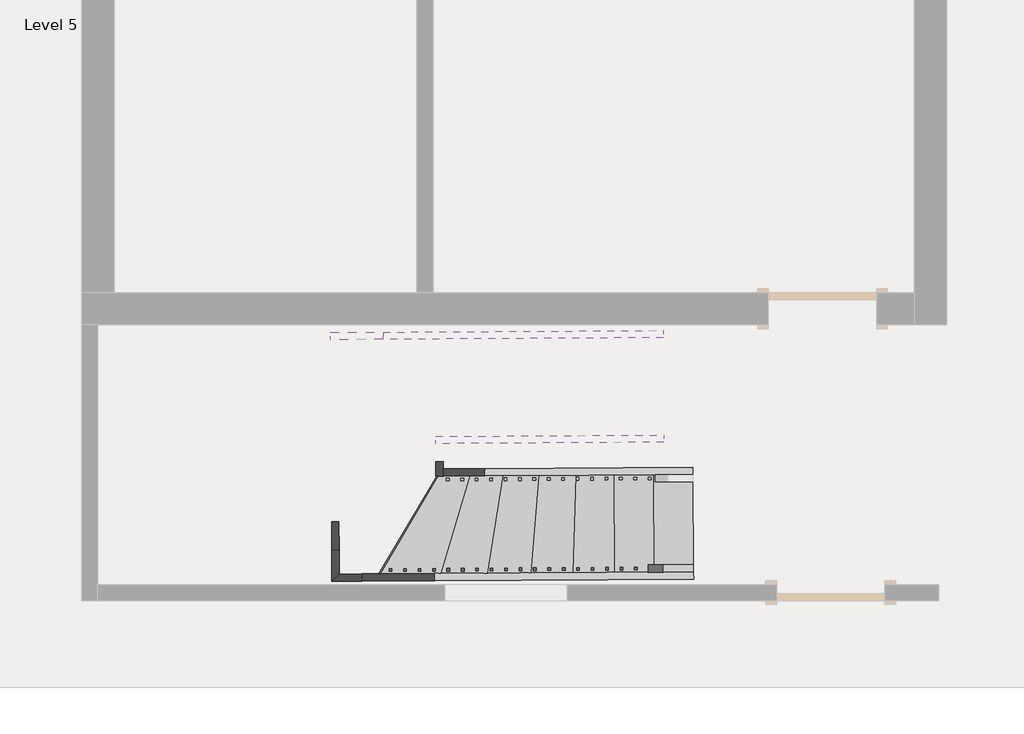
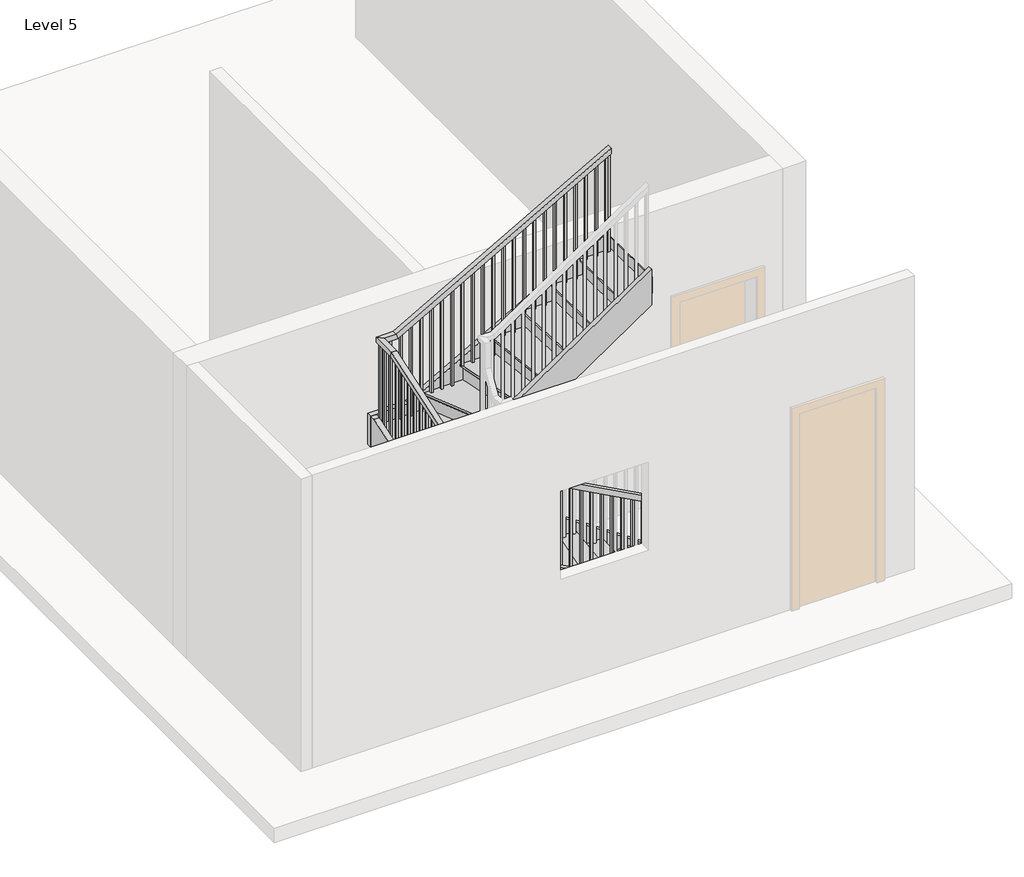
# One storey, part 2 of 2: 9 members, 1 railing, 1 stair flight.
"""IFC4 building model written with IfcOpenShell, lengths in millimetres."""

from ifc_helpers import new_model, si_unit, frame, origin, place, context, project, spatial, polyline, outline, extrude, faceted_brep, transform, mapped, element, save
from components import stair_flight_f68b1b91

model = new_model("IFC4")

# Units and contexts
model_context = context("Model", 3, world=origin())
ifc_project = project(units=[si_unit("LENGTHUNIT", "METRE", prefix="MILLI")], contexts=[model_context])

# Site, building, storey
site = spatial("IfcSite", under=ifc_project)
building = spatial("IfcBuilding", under=site)
storey = spatial("IfcBuildingStorey", under=building, Name="Level 5", Elevation=9601.2)

# Members
placement = place(None, origin())
element("IfcMember", 1, ObjectType="Stringer - 2\" Width", at=placement, inside=storey, context=model_context, shape_type="SweptSolid", body=[
    extrude(outline(polyline([(-106.4787477, -199.0602913), (0.0, 0.0), (2650.4216713, 0.0), (2487.3820108, -304.8), (91.199922, -304.8), (-106.4787477, -199.0602913)])), frame((-116.1777511, -4276.2080688, 9826.9492487), z_axis=(-0.006129891180436152, 0.9999812120405644, 0.0), x_axis=(-0.881759529662862, -0.005405191516664865, 0.4716682263555568)), (0.0, 0.0, 1.0), 50.8),
])
element("IfcMember", 2, ObjectType="Stringer - 2\" Width", at=placement, inside=storey, context=model_context, shape_type="SweptSolid", body=[
    extrude(outline(polyline([(-2453.5237158, -4239.7350599), (-2453.2123174, -4290.5341055), (-2663.1420684, -4291.8209762), (-2612.6544213, -4240.7105322), (-2453.5237158, -4239.7350599)])), frame((0.0, 0.0, 10731.4029558), z_axis=(0.0, 0.0, 1.0), x_axis=(1.0, 0.0, 0.0)), (0.0, 0.0, 1.0), 345.6659817),
])
element("IfcMember", 3, ObjectType="Stringer - 2\" Width", at=placement, inside=storey, context=model_context, shape_type="SweptSolid", body=[
    extrude(outline(polyline([(-2612.6544213, -4240.7105322), (-2663.1420684, -4291.8209762), (-2664.4731567, -4074.6779247), (-2613.6741111, -4074.3665263), (-2612.6544213, -4240.7105322)])), frame((0.0, 0.0, 10731.4029558), z_axis=(0.0, 0.0, 1.0), x_axis=(1.0, 0.0, 0.0)), (0.0, 0.0, 1.0), 345.6659817),
])
element("IfcMember", 4, ObjectType="Stringer - 2\" Width", at=placement, inside=storey, context=model_context, shape_type="SweptSolid", body=[
    extrude(outline(polyline([(-112.9595567, -326.688092), (0.0, 0.0), (1516.7940002, 1e-07), (1565.1210838, -16.7101466), (1457.9394259, -326.6880919), (-112.9595567, -326.688092)])), frame((-2664.4731567, -4074.6779247, 11077.0689375), z_axis=(0.9999812120405643, 0.006129891180436421, 0.0), x_axis=(-0.005793345483301546, 0.9450798501367781, 0.3267881791215163)), (0.0, 0.0, 1.0), 50.8),
])
element("IfcMember", 5, ObjectType="Stringer - 2\" Width", at=placement, inside=storey, context=model_context, shape_type="SweptSolid", body=[
    extrude(outline(polyline([(-111.800968, -163.7049666), (0.0, 0.0), (2130.8093531, 0.0), (1922.648686, -304.8000001), (94.7979387, -304.8000001), (-111.800968, -163.7049666)])), frame((-120.6930289, -3539.621908, 9799.4391801), z_axis=(-0.006129891180436334, 0.9999812120405643, 0.0), x_axis=(-0.8257797012408892, -0.005062034812924604, 0.5639700885880922)), (0.0, 0.0, 1.0), 50.8),
])
element("IfcMember", 6, ObjectType="Stringer - 2\" Width", at=placement, inside=storey, context=model_context, shape_type="SweptSolid", body=[
    extrude(outline(polyline([(-476.3090819, -288.3824073), (0.0, 0.0), (441.380003, 0.0), (-62.0453256, -304.8), (-466.3690133, -304.8), (-476.3090819, -288.3824073)])), frame((-1931.0711854, -3550.7195376, 11223.5542381), z_axis=(0.9999812120405644, 0.006129891180436035, 0.0), x_axis=(-0.0031747997513555445, 0.5179113315223277, 0.8554284150806007)), (0.0, 0.0, 1.0), 50.8),
])
element("IfcMember", 7, ObjectType="Stringer - 2\" Width", at=placement, inside=storey, context=model_context, shape_type="SweptSolid", body=[
    extrude(outline(polyline([(205.0123517, -304.8), (0.0, 0.0), (1938.1040339, 0.0), (2143.1163855, -304.8), (205.0123517, -304.8)])), frame((-1932.4724786, -3322.1238325, 11268.1006308), z_axis=(-0.006129891180436482, 0.9999812120405644, 0.0), x_axis=(0.8297505463599371, 0.005086376118722323, 0.5581112430271987)), (0.0, 0.0, 1.0), 50.8),
])
element("IfcMember", 8, ObjectType="Stringer - 2\" Width", at=placement, inside=storey, context=model_context, shape_type="SweptSolid", body=[
    extrude(outline(polyline([(-2673.5739172, -2590.0529496), (-2673.8853157, -2539.253904), (-2303.2697085, -2536.982028), (-2302.9583101, -2587.7810735), (-2673.5739172, -2590.0529496)])), frame((0.0, 0.0, 11250.2329153), z_axis=(0.0, 0.0, 1.0), x_axis=(1.0, 0.0, 0.0)), (0.0, 0.0, 1.0), 322.5063717),
])
element("IfcMember", 9, ObjectType="Stringer - 2\" Width", at=placement, inside=storey, context=model_context, shape_type="SweptSolid", body=[
    extrude(outline(polyline([(155.3220552, -282.6400873), (0.0, 0.0), (2252.6037587, 1e-07), (2407.9258139, -282.6400872), (155.3220552, -282.6400873)])), frame((-2302.9583101, -2587.7810735, 11250.2329153), z_axis=(-0.006129891180436272, 0.9999812120405644, 0.0), x_axis=(0.8763695910030255, 0.005372151158450034, 0.4816092606637882)), (0.0, 0.0, 1.0), 50.8),
])

# Railing
element("IfcRailing", 10, ObjectType="Handrail - Rectangular", at=placement, inside=storey, context=model_context, shape_type="SolidModel", body=[
    faceted_brep([(-116.4891496, -4225.4090232, 10684.9333333), (-116.4891496, -4225.4090232, 10627.1022634), (-116.800548, -4174.6099776, 10627.1022634), (-116.800548, -4174.6099776, 10684.9333333), (-2474.2717021, -4239.8622452, 11967.6653479), (-2487.1954725, -4239.941468, 11916.8653479), (-2487.506871, -4189.1424224, 11916.8653479), (-2474.5831006, -4189.0631997, 11967.6653479), (-2612.6544213, -4240.7105322, 11967.6653479), (-2612.6544213, -4240.7105322, 11916.8653479), (-2562.1667742, -4189.6000881, 11916.8653479), (-2562.1667742, -4189.6000881, 11967.6653479), (-2613.899826, -4037.5452114, 11967.6653479), (-2613.9521428, -4029.010664, 11916.8653479), (-2563.1530973, -4028.6992655, 11916.8653479), (-2563.1007804, -4037.2338129, 11967.6653479), (-2621.180916, -2849.7666717, 12378.3734867), (-2621.2332328, -2841.2321243, 12327.5734867), (-2570.4341872, -2840.9207258, 12327.5734867), (-2570.3818704, -2849.4552732, 12378.3734867), (-2622.7748716, -2589.7415511, 12378.3734867), (-2622.7748716, -2589.7415511, 12327.5734867), (-2571.6644276, -2640.2291982, 12327.5734867), (-2571.6644276, -2640.2291982, 12378.3734867), (-2452.0429693, -2588.6949634, 12378.3734867), (-2438.8245474, -2588.6139344, 12327.5734867), (-2438.513149, -2639.41298, 12327.5734867), (-2451.7315708, -2639.494009, 12378.3734867), (-328.8448754, -2575.6797456, 13563.6), (-328.533477, -2626.4787912, 13563.6), (-328.533477, -2626.4787912, 13505.42112), (-328.8448754, -2575.6797456, 13505.42112)], [[[0, 1, 2, 3]], [[1, 0, 4, 5]], [[2, 1, 5, 6]], [[3, 2, 6, 7]], [[0, 3, 7, 4]], [[5, 4, 8, 9]], [[6, 5, 9, 10]], [[7, 6, 10, 11]], [[4, 7, 11, 8]], [[9, 8, 12, 13]], [[10, 9, 13, 14]], [[11, 10, 14, 15]], [[8, 11, 15, 12]], [[13, 12, 16, 17]], [[14, 13, 17, 18]], [[15, 14, 18, 19]], [[12, 15, 19, 16]], [[17, 16, 20, 21]], [[18, 17, 21, 22]], [[19, 18, 22, 23]], [[16, 19, 23, 20]], [[21, 20, 24, 25]], [[22, 21, 25, 26]], [[23, 22, 26, 27]], [[20, 23, 27, 24]], [[28, 29, 30, 31]], [[25, 24, 28, 31]], [[26, 25, 31, 30]], [[27, 26, 30, 29]], [[24, 27, 29, 28]]]),
    extrude(outline(polyline([(233.9170124, 19.05), (1235.5250403, 19.05), (1235.5250403, 0.0), (223.2829877, 0.0), (233.9170124, 19.05)])), frame((-352.4784362, -2610.7502757, 13715.391707), z_axis=(-0.0061298911804362555, 0.9999812120405644, 0.0), x_axis=(0.0, 0.0, -1.0)), (0.0, 0.0, 1.0), 19.05),
    extrude(outline(polyline([(233.9170123, 19.05), (1178.8102421, 19.05), (1178.8102421, 0.0), (223.2829877, 0.0), (233.9170123, 19.05)])), frame((-454.0765273, -2611.3730726, 13658.6769088), z_axis=(-0.0061298911804362555, 0.9999812120405644, 0.0), x_axis=(0.0, 0.0, -1.0)), (0.0, 0.0, 1.0), 19.05),
    extrude(outline(polyline([(233.9170124, 19.05), (1122.095444, 19.05), (1122.095444, 0.0), (223.2829877, 0.0), (233.9170124, 19.05)])), frame((-555.6746185, -2611.9958696, 13601.9621107), z_axis=(-0.0061298911804362555, 0.9999812120405644, 0.0), x_axis=(0.0, 0.0, -1.0)), (0.0, 0.0, 1.0), 19.05),
    extrude(outline(polyline([(233.9170123, 19.05), (1234.7139792, 19.05), (1234.7139792, 0.0), (223.2829877, 0.0), (233.9170123, 19.05)])), frame((-657.2727096, -2612.6186665, 13545.2473125), z_axis=(-0.0061298911804362555, 0.9999812120405644, 0.0), x_axis=(0.0, 0.0, -1.0)), (0.0, 0.0, 1.0), 19.05),
    extrude(outline(polyline([(233.9170123, 19.05), (1177.999181, 19.05), (1177.999181, 0.0), (223.2829876, 0.0), (233.9170123, 19.05)])), frame((-758.8708008, -2613.2414635, 13488.5325143), z_axis=(-0.0061298911804362555, 0.9999812120405644, 0.0), x_axis=(0.0, 0.0, -1.0)), (0.0, 0.0, 1.0), 19.05),
    extrude(outline(polyline([(233.9170123, 19.05), (1121.2843829, 19.05), (1121.2843829, 0.0), (223.2829877, 0.0), (233.9170123, 19.05)])), frame((-860.4688919, -2613.8642604, 13431.8177162), z_axis=(-0.0061298911804362555, 0.9999812120405644, 0.0), x_axis=(0.0, 0.0, -1.0)), (0.0, 0.0, 1.0), 19.05),
    extrude(outline(polyline([(233.9170123, 19.0499999), (1233.902918, 19.0499999), (1233.902918, 0.0), (223.2829876, 0.0), (233.9170123, 19.0499999)])), frame((-962.0669831, -2614.4870574, 13375.102918), z_axis=(-0.0061298911804362555, 0.9999812120405644, 0.0), x_axis=(0.0, 0.0, -1.0)), (0.0, 0.0, 1.0), 19.05),
    extrude(outline(polyline([(233.9170123, 19.05), (1177.1881199, 19.05), (1177.1881199, 0.0), (223.2829877, 0.0), (233.9170123, 19.05)])), frame((-1063.6650742, -2615.1098543, 13318.3881199), z_axis=(-0.0061298911804362555, 0.9999812120405644, 0.0), x_axis=(0.0, 0.0, -1.0)), (0.0, 0.0, 1.0), 19.05),
    extrude(outline(polyline([(233.9170123, 19.05), (1120.4733217, 19.05), (1120.4733217, 0.0), (223.2829876, 0.0), (233.9170123, 19.05)])), frame((-1165.2631653, -2615.7326513, 13261.6733217), z_axis=(-0.0061298911804362555, 0.9999812120405644, 0.0), x_axis=(0.0, 0.0, -1.0)), (0.0, 0.0, 1.0), 19.05),
    extrude(outline(polyline([(233.9170123, 19.05), (1233.0918569, 19.05), (1233.0918569, 0.0), (223.2829877, 0.0), (233.9170123, 19.05)])), frame((-1266.8612565, -2616.3554482, 13204.9585236), z_axis=(-0.0061298911804362555, 0.9999812120405644, 0.0), x_axis=(0.0, 0.0, -1.0)), (0.0, 0.0, 1.0), 19.05),
    extrude(outline(polyline([(233.9170123, 19.05), (1176.3770587, 19.05), (1176.3770587, 0.0), (223.2829876, 0.0), (233.9170123, 19.05)])), frame((-1368.4593476, -2616.9782451, 13148.2437254), z_axis=(-0.0061298911804362555, 0.9999812120405644, 0.0), x_axis=(0.0, 0.0, -1.0)), (0.0, 0.0, 1.0), 19.05),
    extrude(outline(polyline([(233.9170123, 19.05), (1288.995594, 19.05), (1288.995594, 0.0), (223.2829877, 0.0), (233.9170123, 19.05)])), frame((-1470.0574388, -2617.6010421, 13091.5289273), z_axis=(-0.0061298911804362555, 0.9999812120405644, 0.0), x_axis=(0.0, 0.0, -1.0)), (0.0, 0.0, 1.0), 19.05),
    extrude(outline(polyline([(233.9170123, 19.05), (1232.2807958, 19.05), (1232.2807958, 0.0), (223.2829876, 0.0), (233.9170123, 19.05)])), frame((-1571.6555299, -2618.223839, 13034.8141291), z_axis=(-0.0061298911804362555, 0.9999812120405644, 0.0), x_axis=(0.0, 0.0, -1.0)), (0.0, 0.0, 1.0), 19.05),
    extrude(outline(polyline([(233.9170123, 19.05), (1175.5659977, 19.05), (1175.5659977, 0.0), (223.2829877, 0.0), (233.9170123, 19.05)])), frame((-1673.2536211, -2618.846636, 12978.099331), z_axis=(-0.0061298911804362555, 0.9999812120405644, 0.0), x_axis=(0.0, 0.0, -1.0)), (0.0, 0.0, 1.0), 19.05),
    extrude(outline(polyline([(233.9170123, 19.05), (1118.8511995, 19.05), (1118.8511995, 0.0), (223.2829876, 0.0), (233.9170123, 19.05)])), frame((-1774.8517122, -2619.4694329, 12921.3845328), z_axis=(-0.0061298911804362555, 0.9999812120405644, 0.0), x_axis=(0.0, 0.0, -1.0)), (0.0, 0.0, 1.0), 19.05),
    extrude(outline(polyline([(233.9170123, 19.05), (1231.4697347, 19.05), (1231.4697347, 0.0), (223.2829877, 0.0), (233.9170123, 19.05)])), frame((-1876.4498033, -2620.0922299, 12864.6697347), z_axis=(-0.0061298911804362555, 0.9999812120405644, 0.0), x_axis=(0.0, 0.0, -1.0)), (0.0, 0.0, 1.0), 19.05),
    extrude(outline(polyline([(233.9170123, 19.05), (1174.7549365, 19.05), (1174.7549365, 0.0), (223.2829876, 0.0), (233.9170123, 19.05)])), frame((-1978.0478945, -2620.7150268, 12807.9549365), z_axis=(-0.0061298911804362555, 0.9999812120405644, 0.0), x_axis=(0.0, 0.0, -1.0)), (0.0, 0.0, 1.0), 19.05),
    extrude(outline(polyline([(233.9170124, 19.05), (1118.0401384, 19.05), (1118.0401384, 0.0), (223.2829877, 0.0), (233.9170124, 19.05)])), frame((-2079.6459856, -2621.3378238, 12751.2401384), z_axis=(-0.0061298911804362555, 0.9999812120405644, 0.0), x_axis=(0.0, 0.0, -1.0)), (0.0, 0.0, 1.0), 19.05),
    extrude(outline(polyline([(233.9170123, 19.05), (1230.6586735, 19.05), (1230.6586735, 0.0), (223.2829876, 0.0), (233.9170123, 19.05)])), frame((-2181.2440768, -2621.9606207, 12694.5253402), z_axis=(-0.0061298911804362555, 0.9999812120405644, 0.0), x_axis=(0.0, 0.0, -1.0)), (0.0, 0.0, 1.0), 19.05),
    extrude(outline(polyline([(233.9170124, 19.05), (1173.9438754, 19.05), (1173.9438754, 0.0), (223.2829877, 0.0), (233.9170124, 19.05)])), frame((-2282.8421679, -2622.5834176, 12637.8105421), z_axis=(-0.0061298911804362555, 0.9999812120405644, 0.0), x_axis=(0.0, 0.0, -1.0)), (0.0, 0.0, 1.0), 19.05),
    extrude(outline(polyline([(233.9170123, 19.05), (1117.2290772, 19.05), (1117.2290772, 0.0), (223.2829877, 0.0), (233.9170123, 19.05)])), frame((-2384.4402591, -2623.2062146, 12581.0957439), z_axis=(-0.0061298911804362555, 0.9999812120405644, 0.0), x_axis=(0.0, 0.0, -1.0)), (0.0, 0.0, 1.0), 19.05),
    extrude(outline(polyline([(-2505.2047667, -2604.8961439), (-2486.1551246, -2604.7793694), (-2486.0383502, -2623.8290115), (-2505.0879923, -2623.945786), (-2505.2047667, -2604.8961439)])), frame((0.0, 0.0, 11463.8666667), z_axis=(0.0, 0.0, 1.0), x_axis=(1.0, 0.0, 0.0)), (0.0, 0.0, 1.0), 863.70682),
    extrude(outline(polyline([(-2606.2189857, -2700.7671513), (-2606.3357602, -2681.7175092), (-2587.2861181, -2681.6007347), (-2587.1693436, -2700.6503768), (-2606.2189857, -2700.7671513)])), frame((0.0, 0.0, 11463.8666667), z_axis=(0.0, 0.0, 1.0), x_axis=(1.0, 0.0, 0.0)), (0.0, 0.0, 1.0), 863.70682),
    extrude(outline(polyline([(-2605.5961888, -2802.3652424), (-2605.7129632, -2783.3156003), (-2586.6633211, -2783.1988259), (-2586.5465467, -2802.248468), (-2605.5961888, -2802.3652424)])), frame((0.0, 0.0, 11463.8666667), z_axis=(0.0, 0.0, 1.0), x_axis=(1.0, 0.0, 0.0)), (0.0, 0.0, 1.0), 863.70682),
    extrude(outline(polyline([(225.3065228, 19.0499999), (1243.2088863, 19.0499999), (1243.2088863, 0.0), (231.8934772, 0.0), (225.3065228, 19.0499999)])), frame((-2604.9733918, -2903.9633335, 12537.7422196), z_axis=(0.9999812120405643, 0.0061298911804362685, 0.0), x_axis=(0.0, 0.0, -1.0)), (0.0, 0.0, 1.0), 19.05),
    extrude(outline(polyline([(225.3065229, 19.05), (1208.078463, 19.05), (1208.078463, 0.0), (231.8934772, 0.0), (225.3065229, 19.05)])), frame((-2604.3505949, -3005.5614247, 12502.6117963), z_axis=(0.9999812120405643, 0.0061298911804362685, 0.0), x_axis=(0.0, 0.0, -1.0)), (0.0, 0.0, 1.0), 19.05),
    extrude(outline(polyline([(225.3065228, 19.05), (1172.9480396, 19.05), (1172.9480396, 0.0), (231.8934772, 0.0), (225.3065228, 19.05)])), frame((-2603.727798, -3107.1595158, 12467.4813729), z_axis=(0.9999812120405643, 0.0061298911804362685, 0.0), x_axis=(0.0, 0.0, -1.0)), (0.0, 0.0, 1.0), 19.05),
    extrude(outline(polyline([(225.3065228, 19.05), (1137.8176163, 19.05), (1137.8176163, 0.0), (231.8934772, 0.0), (225.3065228, 19.05)])), frame((-2603.105001, -3208.757607, 12432.3509496), z_axis=(0.9999812120405643, 0.0061298911804362685, 0.0), x_axis=(0.0, 0.0, -1.0)), (0.0, 0.0, 1.0), 19.05),
    extrude(outline(polyline([(225.3065228, 19.05), (1102.687193, 19.05), (1102.687193, 0.0), (231.8934772, 0.0), (225.3065228, 19.05)])), frame((-2602.4822041, -3310.3556981, 12397.2205263), z_axis=(0.9999812120405643, 0.0061298911804362685, 0.0), x_axis=(0.0, 0.0, -1.0)), (0.0, 0.0, 1.0), 19.05),
    extrude(outline(polyline([(225.3065228, 19.05), (1236.890103, 19.05), (1236.890103, 0.0), (231.8934772, 0.0), (225.3065228, 19.05)])), frame((-2601.8594071, -3411.9537893, 12362.090103), z_axis=(0.9999812120405643, 0.0061298911804362685, 0.0), x_axis=(0.0, 0.0, -1.0)), (0.0, 0.0, 1.0), 19.05),
    extrude(outline(polyline([(225.3065229, 19.05), (1201.7596797, 19.05), (1201.7596797, 0.0), (231.8934772, 0.0), (225.3065229, 19.05)])), frame((-2601.2366102, -3513.5518804, 12326.9596797), z_axis=(0.9999812120405643, 0.0061298911804362685, 0.0), x_axis=(0.0, 0.0, -1.0)), (0.0, 0.0, 1.0), 19.05),
    extrude(outline(polyline([(225.3065228, 19.0499999), (1166.6292563, 19.0499999), (1166.6292563, 0.0), (231.8934772, 0.0), (225.3065228, 19.0499999)])), frame((-2600.6138132, -3615.1499715, 12291.8292563), z_axis=(0.9999812120405643, 0.0061298911804362685, 0.0), x_axis=(0.0, 0.0, -1.0)), (0.0, 0.0, 1.0), 19.05),
    extrude(outline(polyline([(225.3065228, 19.05), (1131.498833, 19.05), (1131.498833, 0.0), (231.8934772, 0.0), (225.3065228, 19.05)])), frame((-2599.9910163, -3716.7480627, 12256.698833), z_axis=(0.9999812120405643, 0.0061298911804362685, 0.0), x_axis=(0.0, 0.0, -1.0)), (0.0, 0.0, 1.0), 19.05),
    extrude(outline(polyline([(225.3065228, 19.05), (1096.3684097, 19.05), (1096.3684097, 0.0), (231.8934772, 0.0), (225.3065228, 19.05)])), frame((-2599.3682194, -3818.3461538, 12221.5684097), z_axis=(0.9999812120405643, 0.0061298911804362685, 0.0), x_axis=(0.0, 0.0, -1.0)), (0.0, 0.0, 1.0), 19.05),
    extrude(outline(polyline([(225.3065228, 19.05), (1230.5713197, 19.05), (1230.5713197, 0.0), (231.8934772, 0.0), (225.3065228, 19.05)])), frame((-2598.7454224, -3919.944245, 12186.4379864), z_axis=(0.9999812120405643, 0.0061298911804362685, 0.0), x_axis=(0.0, 0.0, -1.0)), (0.0, 0.0, 1.0), 19.05),
    extrude(outline(polyline([(225.3065228, 19.05), (1195.4408963, 19.05), (1195.4408963, 0.0), (231.8934771, 0.0), (225.3065228, 19.05)])), frame((-2598.1226255, -4021.5423361, 12151.307563), z_axis=(0.9999812120405643, 0.0061298911804362685, 0.0), x_axis=(0.0, 0.0, -1.0)), (0.0, 0.0, 1.0), 19.05),
    extrude(outline(polyline([(-2597.4998285, -4123.1404273), (-2597.6166029, -4104.0907852), (-2578.5669609, -4103.9740107), (-2578.4501864, -4123.0236528), (-2597.4998285, -4123.1404273)])), frame((0.0, 0.0, 10955.8666667), z_axis=(0.0, 0.0, 1.0), x_axis=(1.0, 0.0, 0.0)), (0.0, 0.0, 1.0), 960.9986813),
    extrude(outline(polyline([(-2545.415828, -4224.4230609), (-2564.4654701, -4224.5398353), (-2564.5822445, -4205.4901932), (-2545.5326024, -4205.3734188), (-2545.415828, -4224.4230609)])), frame((0.0, 0.0, 10955.8666667), z_axis=(0.0, 0.0, 1.0), x_axis=(1.0, 0.0, 0.0)), (0.0, 0.0, 1.0), 960.9986813),
    extrude(outline(polyline([(223.4181002, 19.05), (1171.1283424, 19.05), (1171.1283424, 0.0), (233.7818998, 0.0), (223.4181002, 19.05)])), frame((-2443.8177368, -4223.800264, 12126.9950091), z_axis=(-0.006129891180436165, 0.9999812120405643, 0.0), x_axis=(0.0, 0.0, -1.0)), (0.0, 0.0, 1.0), 19.05),
    extrude(outline(polyline([(223.4181002, 19.05), (1115.8547448, 19.05), (1115.8547448, 0.0), (233.7818998, 0.0), (223.4181002, 19.05)])), frame((-2342.2196457, -4223.177467, 12071.7214115), z_axis=(-0.006129891180436165, 0.9999812120405643, 0.0), x_axis=(0.0, 0.0, -1.0)), (0.0, 0.0, 1.0), 19.05),
    extrude(outline(polyline([(223.4181002, 19.05), (1229.9144805, 19.05), (1229.9144805, 0.0), (233.7818997, 0.0), (223.4181002, 19.05)])), frame((-2240.6215545, -4222.5546701, 12016.4478138), z_axis=(-0.006129891180436165, 0.9999812120405643, 0.0), x_axis=(0.0, 0.0, -1.0)), (0.0, 0.0, 1.0), 19.05),
    extrude(outline(polyline([(223.4181002, 19.05), (1174.6408829, 19.05), (1174.6408829, 0.0), (233.7818998, 0.0), (223.4181002, 19.05)])), frame((-2139.0234634, -4221.9318731, 11961.1742162), z_axis=(-0.006129891180436165, 0.9999812120405643, 0.0), x_axis=(0.0, 0.0, -1.0)), (0.0, 0.0, 1.0), 19.05),
    extrude(outline(polyline([(223.4181003, 19.0499999), (1119.3672853, 19.0499999), (1119.3672853, 0.0), (233.7818998, 0.0), (223.4181003, 19.0499999)])), frame((-2037.4253723, -4221.3090762, 11905.9006186), z_axis=(-0.006129891180436165, 0.9999812120405643, 0.0), x_axis=(0.0, 0.0, -1.0)), (0.0, 0.0, 1.0), 19.05),
    extrude(outline(polyline([(223.4181002, 19.05), (1064.0936876, 19.05), (1064.0936876, 0.0), (233.7818998, 0.0), (223.4181002, 19.05)])), frame((-1935.8272811, -4220.6862792, 11850.6270209), z_axis=(-0.006129891180436165, 0.9999812120405643, 0.0), x_axis=(0.0, 0.0, -1.0)), (0.0, 0.0, 1.0), 19.05),
    extrude(outline(polyline([(223.4181002, 19.05), (1178.1534233, 19.05), (1178.1534233, 0.0), (233.7818998, 0.0), (223.4181002, 19.05)])), frame((-1834.22919, -4220.0634823, 11795.3534233), z_axis=(-0.006129891180436165, 0.9999812120405643, 0.0), x_axis=(0.0, 0.0, -1.0)), (0.0, 0.0, 1.0), 19.05),
    extrude(outline(polyline([(223.4181002, 19.05), (1122.8798256, 19.05), (1122.8798256, 0.0), (233.7818997, 0.0), (223.4181002, 19.05)])), frame((-1732.6310988, -4219.4406854, 11740.0798256), z_axis=(-0.006129891180436165, 0.9999812120405643, 0.0), x_axis=(0.0, 0.0, -1.0)), (0.0, 0.0, 1.0), 19.05),
    extrude(outline(polyline([(223.4181002, 19.05), (1067.606228, 19.05), (1067.606228, 0.0), (233.7818998, 0.0), (223.4181002, 19.05)])), frame((-1631.0330077, -4218.8178884, 11684.806228), z_axis=(-0.006129891180436165, 0.9999812120405643, 0.0), x_axis=(0.0, 0.0, -1.0)), (0.0, 0.0, 1.0), 19.05),
    extrude(outline(polyline([(223.4181003, 19.05), (1181.6659637, 19.05), (1181.6659637, 0.0), (233.7818998, 0.0), (223.4181003, 19.05)])), frame((-1529.4349165, -4218.1950915, 11629.5326304), z_axis=(-0.006129891180436165, 0.9999812120405643, 0.0), x_axis=(0.0, 0.0, -1.0)), (0.0, 0.0, 1.0), 19.05),
    extrude(outline(polyline([(223.4181002, 19.05), (1126.392366, 19.05), (1126.392366, 0.0), (233.7818998, 0.0), (223.4181002, 19.05)])), frame((-1427.8368254, -4217.5722945, 11574.2590327), z_axis=(-0.006129891180436165, 0.9999812120405643, 0.0), x_axis=(0.0, 0.0, -1.0)), (0.0, 0.0, 1.0), 19.05),
    extrude(outline(polyline([(223.4181002, 19.0499999), (1071.1187684, 19.0499999), (1071.1187684, 0.0), (233.7818998, 0.0), (223.4181002, 19.0499999)])), frame((-1326.2387343, -4216.9494976, 11518.9854351), z_axis=(-0.006129891180436165, 0.9999812120405643, 0.0), x_axis=(0.0, 0.0, -1.0)), (0.0, 0.0, 1.0), 19.05),
    extrude(outline(polyline([(223.4181002, 19.05), (1185.1785041, 19.05), (1185.1785041, 0.0), (233.7818997, 0.0), (223.4181002, 19.05)])), frame((-1224.6406431, -4216.3267006, 11463.7118374), z_axis=(-0.006129891180436165, 0.9999812120405643, 0.0), x_axis=(0.0, 0.0, -1.0)), (0.0, 0.0, 1.0), 19.05),
    extrude(outline(polyline([(223.4181002, 19.05), (1129.9049065, 19.05), (1129.9049065, 0.0), (233.7818998, 0.0), (223.4181002, 19.05)])), frame((-1123.042552, -4215.7039037, 11408.4382398), z_axis=(-0.006129891180436165, 0.9999812120405643, 0.0), x_axis=(0.0, 0.0, -1.0)), (0.0, 0.0, 1.0), 19.05),
    extrude(outline(polyline([(223.4181003, 19.05), (1074.6313089, 19.05), (1074.6313089, 0.0), (233.7818998, 0.0), (223.4181003, 19.05)])), frame((-1021.4444608, -4215.0811067, 11353.1646422), z_axis=(-0.006129891180436165, 0.9999812120405643, 0.0), x_axis=(0.0, 0.0, -1.0)), (0.0, 0.0, 1.0), 19.05),
    extrude(outline(polyline([(223.4181002, 19.05), (1188.6910445, 19.05), (1188.6910445, 0.0), (233.7818998, 0.0), (223.4181002, 19.05)])), frame((-919.8463697, -4214.4583098, 11297.8910445), z_axis=(-0.006129891180436165, 0.9999812120405643, 0.0), x_axis=(0.0, 0.0, -1.0)), (0.0, 0.0, 1.0), 19.05),
    extrude(outline(polyline([(223.4181002, 19.05), (1133.4174469, 19.05), (1133.4174469, 0.0), (233.7818998, 0.0), (223.4181002, 19.05)])), frame((-818.2482785, -4213.8355129, 11242.6174469), z_axis=(-0.006129891180436165, 0.9999812120405643, 0.0), x_axis=(0.0, 0.0, -1.0)), (0.0, 0.0, 1.0), 19.05),
    extrude(outline(polyline([(223.4181002, 19.05), (1078.1438492, 19.05), (1078.1438492, 0.0), (233.7818997, 0.0), (223.4181002, 19.05)])), frame((-716.6501874, -4213.2127159, 11187.3438492), z_axis=(-0.006129891180436165, 0.9999812120405643, 0.0), x_axis=(0.0, 0.0, -1.0)), (0.0, 0.0, 1.0), 19.05),
    extrude(outline(polyline([(223.4181002, 19.0499999), (1192.2035849, 19.0499999), (1192.2035849, 0.0), (233.7818998, 0.0), (223.4181002, 19.0499999)])), frame((-615.0520963, -4212.589919, 11132.0702516), z_axis=(-0.006129891180436165, 0.9999812120405643, 0.0), x_axis=(0.0, 0.0, -1.0)), (0.0, 0.0, 1.0), 19.05),
    extrude(outline(polyline([(223.4181003, 19.05), (1136.9299873, 19.05), (1136.9299873, 0.0), (233.7818998, 0.0), (223.4181003, 19.05)])), frame((-513.4540051, -4211.967122, 11076.796654), z_axis=(-0.006129891180436165, 0.9999812120405643, 0.0), x_axis=(0.0, 0.0, -1.0)), (0.0, 0.0, 1.0), 19.05),
    extrude(outline(polyline([(223.4181002, 19.05), (1081.6563896, 19.05), (1081.6563896, 0.0), (233.7818998, 0.0), (223.4181002, 19.05)])), frame((-411.855914, -4211.3443251, 11021.5230563), z_axis=(-0.006129891180436165, 0.9999812120405643, 0.0), x_axis=(0.0, 0.0, -1.0)), (0.0, 0.0, 1.0), 19.05),
    extrude(outline(polyline([(223.4181002, 19.05), (1195.7161254, 19.05), (1195.7161254, 0.0), (233.7818998, 0.0), (223.4181002, 19.05)])), frame((-310.2578228, -4210.7215281, 10966.2494587), z_axis=(-0.006129891180436165, 0.9999812120405643, 0.0), x_axis=(0.0, 0.0, -1.0)), (0.0, 0.0, 1.0), 19.05),
    extrude(outline(polyline([(223.4181002, 19.05), (1140.4425277, 19.05), (1140.4425277, 0.0), (233.7818997, 0.0), (223.4181002, 19.05)])), frame((-208.6597317, -4210.0987312, 10910.975861), z_axis=(-0.006129891180436165, 0.9999812120405643, 0.0), x_axis=(0.0, 0.0, -1.0)), (0.0, 0.0, 1.0), 19.05),
    extrude(outline(polyline([(-2606.6860834, -2624.5685829), (-2606.8028579, -2605.5189408), (-2587.7532158, -2605.4021664), (-2587.6364414, -2624.4518085), (-2606.6860834, -2624.5685829)])), frame((0.0, 0.0, 11463.8666667), z_axis=(0.0, 0.0, 1.0), x_axis=(1.0, 0.0, 0.0)), (0.0, 0.0, 1.0), 863.70682),
    extrude(outline(polyline([(-2577.8273895, -4224.621744), (-2596.8770316, -4224.7385184), (-2596.993806, -4205.6888763), (-2577.9441639, -4205.5721019), (-2577.8273895, -4224.621744)])), frame((0.0, 0.0, 10955.8666667), z_axis=(0.0, 0.0, 1.0), x_axis=(1.0, 0.0, 0.0)), (0.0, 0.0, 1.0), 960.9986813),
    extrude(outline(polyline([(233.9170123, 19.05), (1248.8374409, 19.05), (1248.8374409, 0.0), (223.2829876, 0.0), (233.9170123, 19.05)])), frame((-328.630789, -2610.6040895, 13728.7041076), z_axis=(-0.0061298911804362555, 0.9999812120405644, 0.0), x_axis=(0.0, 0.0, -1.0)), (0.0, 0.0, 1.0), 19.05),
    extrude(outline(polyline([(223.4181002, 19.05), (1090.3508299, 19.05), (1090.3508299, 0.0), (233.7818998, 0.0), (223.4181002, 19.05)])), frame((-116.5864616, -4209.5343215, 10860.8841632), z_axis=(-0.006129891180436165, 0.9999812120405643, 0.0), x_axis=(0.0, 0.0, -1.0)), (0.0, 0.0, 1.0), 19.05),
])

# Stair flight
stair_flight_shape = stair_flight_f68b1b91(model_context)
element("IfcStairFlight", 11, ObjectType="2\" Tread 1\" Nosing 1/4\" Riser", at=placement, inside=storey, context=model_context, shape_type="MappedRepresentation", body=[
    mapped(stair_flight_shape, transform((0.0, 0.0, 0.0), x_axis=(1.0, 0.0, 0.0), y_axis=(0.0, 1.0, 0.0), z_axis=(0.0, 0.0, 1.0))),
])

save(model, "model.ifc")

# Revit data of these elements
# Type "Handrail - Rectangular"
#   Assembly Code = "C2010400"
#   built-in parameter 1008612 = 0.0416667 (stored number, unit not read)
#   built-in parameter 1008611 = 0.0416667 (stored number, unit not read)
#   built-in parameter 1008609 = 0.333333 (stored number, unit not read)
#   built-in parameter 1008604 = 0.166667 (stored number, unit not read)
#   built-in parameter 1008603 = 0.166667 (stored number, unit not read)
#   Railing Height = 3' - 0"
#   built-in parameter 1008630 = 2
#   built-in parameter 1008610 = 2
#   built-in parameter 1008618 = Baluster - Square : 3/4"
# Elements 1, 2, 3, 4, 5, 6, 7, 8, 9 (IfcMember, "Stringer - 2\" Width")
#   Phase Created = New Construction
# Element 10 (IfcRailing, "Handrail - Rectangular")
#   Phase Created = New Construction
# Element 11 (IfcStairFlight, "2\" Tread 1\" Nosing 1/4\" Riser")
#   Phase Created = New Construction
#   Materials on its faces: "Door - Frame"
# Materials
#   "Door - Frame": colour RGB 118 70 51, transparency 0, Cost = 0
